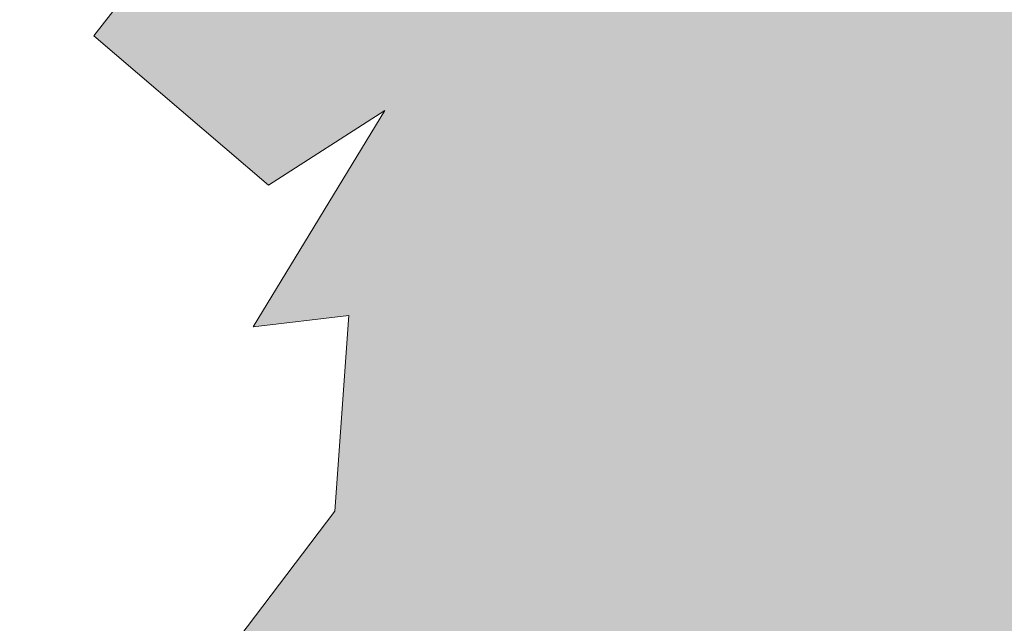
# Model space of a CAD drawing. Units: inches. Extents: x 2091 to 2899, y 967 to 2217.
# Tile 256 of 256: x 2231.62 to 2253.52, y 1152.59 to 1166.02. Entities that reach past the tile are written whole.
import ezdxf

# ---------------------------------------------------------------- set-up
doc = ezdxf.new("R2010")
doc.units = ezdxf.units.IN
doc.layers.add('A-ANNO-DIMS', color=2, linetype='Continuous', lineweight=18)
doc.layers.add('L-PLNT-TREE', color=94, linetype='Continuous', lineweight=13)
doc.layers.add('A-WALL-PATT', color=141, linetype='Continuous', lineweight=13, true_color=0xadddf7)
doc.layers.add('L-PLNT-PATT', color=114, linetype='Continuous', lineweight=13, true_color=0x139b48)
doc.styles.get("Standard").update_dxf_attribs({"font": 'arial.ttf'})
doc.dimstyles.new('ISO-25', dxfattribs={"dimtxt": 4, "dimasz": 4, "dimexe": 1.25, "dimexo": 0.625, "dimtad": 1, "dimdec": 0, "dimlunit": 3, "dimtxsty": 'Standard', "dimcen": 2.5, "dimadec": 0, "dimazin": 0, "dimtfac": 1, "dimtdec": 0, "dimtmove": 0, "dimatfit": 3, "dimfxl": 1, "dimarcsym": 0})

# ---------------------------------------------------------------- blocks, each defined once
blk = doc.blocks.new('*U25')
blk.add_lwpolyline([(-1139.42368, 1783.79628), (-1216.11644, 1685.47796), (-1117.5111, 1601.2033), (-1051.7759, 1643.3419), (-1126.09884, 1521.20092), (-1072.10606, 1527.49758), (-1079.90386, 1416.93646), (-1259.93906, 1179.83508), (-1479.05978, 1165.78888), (-1577.66258, 1109.60662), (-1742.00312, 927.01364), (-1676.26538, 814.64658), (-1270.89408, 828.69278), (-1194.20386, 772.51052), (-1007.95074, 856.78518), (-876.4778, 575.87134), (-821.70016, 575.87134), (-569.71184, 884.87504)])
blk = doc.blocks.new('*D71')
at = {"layer": 'A-ANNO-DIMS', "color": 0, "lineweight": -2, "transparency": 16777216}
for p, q in [((2212.144, 1351.294), (2212.144, 969.464)), ((2452.144, 1351.294), (2452.144, 969.464)), ((2216.144, 970.714), (2448.144, 970.714))]:
    blk.add_line(p, q, dxfattribs=at)
at = {"layer": 'A-ANNO-DIMS', "color": 0, "transparency": 16777216}
for points in [[(2216.144, 971.381), (2216.144, 970.048), (2212.144, 970.714)], [(2448.144, 971.381), (2448.144, 970.048), (2452.144, 970.714)]]:
    blk.add_solid(points, dxfattribs=at)
at = {"layer": 'Defpoints', "color": 0, "transparency": 16777216}
for p in [(2212.144, 1351.919), (2452.144, 1351.919), (2452.144, 970.714)]:
    blk.add_point(p, dxfattribs=at)
at = {"layer": 'A-ANNO-DIMS', "color": 0, "transparency": 16777216, "insert": (2332.144, 973.382), "char_height": 4, "attachment_point": 5}
blk.add_mtext('20\'-0"', dxfattribs=at)
blk = doc.blocks.new('*D75')
at = {"layer": 'A-ANNO-DIMS', "color": 0, "lineweight": -2, "transparency": 16777216}
for p, q in [((2212.144, 1274.794), (2212.144, 969.464)), ((2308.144, 1274.794), (2308.144, 969.464)), ((2216.144, 970.714), (2304.144, 970.714))]:
    blk.add_line(p, q, dxfattribs=at)
at = {"layer": 'A-ANNO-DIMS', "color": 0, "transparency": 16777216}
for points in [[(2216.144, 971.381), (2216.144, 970.048), (2212.144, 970.714)], [(2304.144, 971.381), (2304.144, 970.048), (2308.144, 970.714)]]:
    blk.add_solid(points, dxfattribs=at)
at = {"layer": 'Defpoints', "color": 0, "transparency": 16777216}
for p in [(2212.144, 1275.419), (2308.144, 1275.419), (2308.144, 970.714)]:
    blk.add_point(p, dxfattribs=at)
at = {"layer": 'A-ANNO-DIMS', "color": 0, "transparency": 16777216, "insert": (2260.144, 973.382), "char_height": 4, "attachment_point": 5}
blk.add_mtext('8\'-0"', dxfattribs=at)

msp = doc.modelspace()

# ---------------------------------------------------------------- hatches: boundary and pattern name
at = {"layer": 'A-WALL-PATT'}
h = msp.add_hatch(color=256, dxfattribs=at)
h.dxf.hatch_style = 1
h.paths.add_polyline_path([(2803.144, 2050.919), (2203.144, 2050.919), (2203.144, 1090.919), (2803.144, 1090.919)])
h.paths.add_polyline_path([(2635.799, 1147.54), (2674.524, 1147.54, 0.376086), (2678.53, 1152.88), (2678.53, 1159.556, 0.333335), (2674.524, 1163.562), (2674.524, 1163.562), (2674.524, 1192.934), (2635.806, 1192.934), (2597.088, 1192.934), (2597.088, 1163.562, 0.333335), (2593.082, 1159.556), (2593.082, 1152.88, 0.376086), (2597.088, 1147.54)], flags=0)
h.paths.add_polyline_path([(2436.01, 1278.241, 0.000483), (2435.953, 1278.215, -0.001328), (2435.936, 1278.112, -0.001711), (2436.116, 1278.041, 0.002185)], flags=0)
h.paths.add_polyline_path([(2794.144, 1143.419), (2794.144, 1347.419), (2543.37, 1347.419), (2543.37, 1351.919), (2794.144, 1351.919), (2794.144, 1392.714), (2793.947, 1392.714), (2793.947, 1473.537), (2794.144, 1473.537), (2794.144, 1531.919), (2650.144, 1531.919), (2650.144, 1536.419), (2794.144, 1536.419), (2794.144, 1692.419), (2609.376, 1692.419), (2609.376, 1644.419), (2604.876, 1644.419), (2604.876, 1744.919), (2609.376, 1744.919), (2609.376, 1696.919), (2794.144, 1696.919), (2794.144, 1780.919), (2609.644, 1780.919), (2493.876, 1780.919), (2493.876, 1785.419), (2609.644, 1785.419), (2794.144, 1785.419), (2794.144, 1847.939), (2793.951, 1847.939), (2793.951, 1928.762), (2794.144, 1928.762), (2794.144, 1941.419), (2614.144, 1941.419), (2614.144, 1821.419), (2609.644, 1821.419), (2609.644, 1941.419), (2392.144, 1941.419), (2392.144, 1819.919), (2387.644, 1819.919), (2387.644, 1941.419), (2212.144, 1941.419), (2212.144, 1783.919), (2392.144, 1783.919), (2392.144, 1780.919), (2212.144, 1780.919), (2212.144, 1629.419), (2387.644, 1629.419), (2387.644, 1744.919), (2392.144, 1744.919), (2392.144, 1627.919), (2317.144, 1627.919), (2317.144, 1551.419), (2317.144, 1536.419), (2459.384, 1536.419), (2459.384, 1602.396), (2463.884, 1602.396), (2463.884, 1531.919), (2456.644, 1531.919), (2456.644, 1529.919), (2452.144, 1529.919), (2452.144, 1531.919), (2312.644, 1531.919), (2312.644, 1551.419), (2306.144, 1551.419), (2306.144, 1555.919), (2308.144, 1555.919), (2308.144, 1551.419), (2312.644, 1551.419), (2312.644, 1627.919), (2212.144, 1627.919), (2212.144, 1555.919), (2270.144, 1555.919), (2270.144, 1551.419), (2212.144, 1551.419), (2212.144, 1351.919), (2272.144, 1351.919), (2272.144, 1347.419), (2212.144, 1347.419), (2212.144, 1275.419), (2308.144, 1275.419), (2308.144, 1351.919), (2452.144, 1351.919), (2452.144, 1493.919), (2456.644, 1493.919), (2456.644, 1347.419), (2312.644, 1347.419), (2312.644, 1270.919), (2212.144, 1270.919), (2212.144, 1099.919), (2281.238, 1099.919), (2282.871, 1110.914), (2282.008, 1116.997), (2278.558, 1121.42), (2268.206, 1128.056), (2272.088, 1128.056), (2273.813, 1131.927), (2279.42, 1134.692), (2285.028, 1135.245), (2287.616, 1137.457), (2288.047, 1138.01), (2289.341, 1140.775), (2291.067, 1139.669), (2292.361, 1135.245), (2295.38, 1136.904), (2296.243, 1135.798), (2297.105, 1133.033), (2300.125, 1138.01), (2303.144, 1138.01), (2304.438, 1135.798), (2303.144, 1133.586), (2306.595, 1134.692), (2307.889, 1133.033), (2310.908, 1135.245), (2313.927, 1134.139), (2315.627, 1132.427), (2308.32, 1117.55), (2290.204, 1109.808), (2288.91, 1103.172), (2289.272, 1099.919), (2434.918, 1099.919), (2431.593, 1124.788), (2429.93, 1169.553), (2430.927, 1240.52), (2435.659, 1238.186), (2437.135, 1196.554), (2438.798, 1143.973), (2442.678, 1111.998), (2446.558, 1099.919), (2794.144, 1099.919), (2794.144, 1138.919), (2548.032, 1138.919), (2548.032, 1143.419), (2548.032, 1148.819), (2546.668, 1148.032), (2528.686, 1179.179, 0.256256), (2512.032, 1148.819), (2512.032, 1143.419), (2512.032, 1138.919), (2507.532, 1138.919), (2507.532, 1143.419), (2507.532, 1148.819, 0.256256), (2490.879, 1179.179), (2472.896, 1148.032), (2471.532, 1148.819), (2471.532, 1143.419), (2467.032, 1143.419), (2467.032, 1269.946, 0.039061), (2460.91, 1273.58), (2467.032, 1273.58), (2467.032, 1286.325, 0.014511), (2465.216, 1286.762), (2467.032, 1287.053), (2467.032, 1323.419), (2471.532, 1323.419), (2471.532, 1148.819), (2489.532, 1179.996), (2490.896, 1179.208), (2490.879, 1179.179, -0.256256), (2507.532, 1148.819), (2507.532, 1143.419), (2512.032, 1143.419), (2512.032, 1148.819, -0.256256), (2528.686, 1179.179), (2528.668, 1179.208), (2530.032, 1179.996), (2548.032, 1148.819), (2548.032, 1143.419)], flags=16)
h.paths.add_polyline_path([(2607.769, 1200.945), (2607.769, 1265.031), (2597.088, 1281.052), (2619.785, 1281.052), (2627.795, 1337.127), (2635.799, 1337.127), (2643.817, 1337.127), (2651.827, 1281.052), (2674.524, 1281.052), (2663.843, 1265.031), (2663.843, 1200.945), (2635.806, 1200.945)], flags=0)
edge = h.paths.add_edge_path(flags=0)
edge.add_ellipse((13303.896, 1272.999), major_axis=(-10595.313, 0), ratio=0.84230387, start_angle=0.6282372, end_angle=0.6465541, ccw=False)
edge.add_ellipse((2711.7, 1156.853), major_axis=(2.22, 0), ratio=0.842304, start_angle=111.5352, end_angle=180.6282, ccw=False)
edge.add_ellipse((13303.156, 1272.999), major_axis=(-10593.026, 0), ratio=0.84230387, start_angle=0.5282715, end_angle=0.6465541, ccw=False)
edge.add_line((2710.765, 1175.333), (2710.13, 1175.333))
edge.add_ellipse((2710.13, 1176.58), major_axis=(1.48, 0), ratio=0.842304, start_angle=180, end_angle=270, ccw=False)
edge.add_line((2708.65, 1176.58), (2708.65, 1200.783))
edge.add_ellipse((2710.13, 1200.783), major_axis=(1.48, 0), ratio=0.842304, start_angle=90, end_angle=180, ccw=False)
edge.add_line((2710.13, 1202.029), (2710.465, 1202.029))
edge.add_ellipse((13303.156, 1272.999), major_axis=(-10593.026, 0), ratio=0.84230387, start_angle=-0.0902291, end_angle=0.3838668, ccw=False)
edge.add_ellipse((2710.13, 1290.927), major_axis=(-1.48, 0), ratio=0.842304, start_angle=0, end_angle=90, ccw=False)
edge.add_line((2708.65, 1290.927), (2708.65, 1315.13))
edge.add_ellipse((2710.13, 1315.13), major_axis=(-1.48, 0), ratio=0.842304, start_angle=-90, end_angle=0, ccw=False)
edge.add_line((2710.13, 1316.377), (2710.706, 1316.377))
edge.add_ellipse((3238.402, 1296.29), major_axis=(528.234, 0), ratio=0.8423039, start_angle=176.34957, end_angle=177.82005, ccw=False)
edge.add_ellipse((2775.063, 1071.451), major_axis=(313.308, 0), ratio=0.8423039, start_angle=102.12597, end_angle=103.78053, ccw=False)
edge.add_ellipse((2775.063, 1078.306), major_axis=(-305.303, 0), ratio=0.8423039, start_angle=-79.79046, end_angle=-77.55537, ccw=False)
edge.add_ellipse((2695.142, 1541.975), major_axis=(-250.96, 0), ratio=0.8423039, start_angle=99.25657, end_angle=102.55493)
edge.add_line((2741.41, 1334.214), (2747.133, 1337.378))
edge.add_ellipse((2747.539, 1336.857), major_axis=(-0.74, 0), ratio=0.842304, start_angle=270, end_angle=307.9331, ccw=False)
edge.add_ellipse((2747.539, 1336.857), major_axis=(-0.74, 0), ratio=0.842304, start_angle=232.0669, end_angle=270, ccw=False)
edge.add_line((2747.945, 1337.378), (2753.667, 1334.214))
edge.add_ellipse((2799.935, 1541.975), major_axis=(250.96, 0), ratio=0.8423039, start_angle=257.44507, end_angle=260.74343)
edge.add_ellipse((2720.014, 1078.306), major_axis=(305.303, 0), ratio=0.8423039, start_angle=77.55537, end_angle=79.79046, ccw=False)
edge.add_ellipse((2720.014, 1071.451), major_axis=(-313.308, 0), ratio=0.8423039, start_angle=256.21947, end_angle=257.87403, ccw=False)
edge.add_ellipse((2256.676, 1296.29), major_axis=(-528.234, 0), ratio=0.8423039, start_angle=182.17995, end_angle=183.65043, ccw=False)
edge.add_line((2784.371, 1316.377), (2784.947, 1316.377))
edge.add_ellipse((2784.947, 1315.13), major_axis=(1.48, 0), ratio=0.842304, start_angle=0, end_angle=90, ccw=False)
edge.add_line((2786.427, 1315.13), (2786.427, 1290.927))
edge.add_ellipse((2784.947, 1290.927), major_axis=(1.48, 0), ratio=0.842304, start_angle=270, end_angle=360, ccw=False)
edge.add_ellipse((-7808.079, 1272.999), major_axis=(10593.026, 0), ratio=0.84230387, start_angle=-0.3838668, end_angle=0.0902291, ccw=False)
edge.add_line((2784.612, 1202.029), (2784.947, 1202.029))
edge.add_ellipse((2784.947, 1200.783), major_axis=(1.48, 0), ratio=0.842304, start_angle=0, end_angle=90, ccw=False)
edge.add_line((2786.427, 1200.783), (2786.427, 1176.58))
edge.add_ellipse((2784.947, 1176.58), major_axis=(-1.48, 0), ratio=0.842304, start_angle=90, end_angle=180, ccw=False)
edge.add_line((2784.947, 1175.333), (2784.313, 1175.333))
edge.add_ellipse((-7808.079, 1272.999), major_axis=(10593.026, 0), ratio=0.84230387, start_angle=-0.6186432, end_angle=-0.5282715, ccw=False)
edge.add_ellipse((2783.377, 1156.853), major_axis=(-2.22, 0), ratio=0.842304, start_angle=179.3718, end_angle=248.4648, ccw=False)
edge.add_ellipse((-7808.819, 1272.999), major_axis=(-10595.313, 0), ratio=0.842303866, start_angle=179.3534459, end_angle=179.3717628, ccw=False)
edge.add_ellipse((2780.297, 1153.501), major_axis=(-5.246, 0), ratio=0.842304, start_angle=90, end_angle=179.3534, ccw=False)
edge.add_line((2780.297, 1149.082), (2714.78, 1149.082))
edge.add_ellipse((2714.78, 1153.501), major_axis=(5.246, 0), ratio=0.842304, start_angle=180.6466, end_angle=270, ccw=False)
edge = h.paths.add_edge_path(flags=0)
edge.add_line((2718.187, 1151.008), (2718.187, 1170.472))
edge.add_ellipse((2721.147, 1170.472), major_axis=(-2.96, 0), ratio=0.842304, start_angle=-90, end_angle=0, ccw=False)
edge.add_line((2721.147, 1172.965), (2773.93, 1172.965))
edge.add_ellipse((2773.93, 1170.472), major_axis=(-2.96, 0), ratio=0.842304, start_angle=180, end_angle=270, ccw=False)
edge.add_line((2776.89, 1170.472), (2776.89, 1151.008))
edge.add_line((2776.89, 1151.008), (2718.187, 1151.008))
edge = h.paths.add_edge_path(flags=0)
edge.add_line((2718.187, 1180.234), (2718.187, 1199.058))
edge.add_ellipse((2747.539, 1320.399), major_axis=(147.018, 0), ratio=0.8423039, start_angle=256.40187, end_angle=283.59813)
edge.add_line((2776.89, 1199.058), (2776.89, 1180.234))
edge.add_ellipse((2747.539, 1301.575), major_axis=(147.018, 0), ratio=0.8423039, start_angle=256.40187, end_angle=283.59813, ccw=False)
edge = h.paths.add_edge_path(flags=0)
edge.add_ellipse((13303.156, 1272.999), major_axis=(-10591.546, 0), ratio=0.84230387, start_angle=0.0555943, end_angle=0.3777642, ccw=False)
edge.add_line((2711.617, 1262.722), (2715.667, 1249.495))
edge.add_ellipse((6413.892, 1241.692), major_axis=(-3698.236, 0), ratio=0.84230387, start_angle=-0.120897, end_angle=0.364076)
edge.add_line((2715.761, 1218.192), (2711.934, 1203.167))
edge = h.paths.add_edge_path(flags=0)
edge.add_line((2718.187, 1251.075), (2716.002, 1267.45))
edge.add_ellipse((2742.151, 1202.19), major_axis=(81.773, 0), ratio=0.842304, start_angle=94.27742, end_angle=111.83495, ccw=False)
edge.add_line((2737.01, 1270.931), (2758.067, 1270.931))
edge.add_ellipse((2752.926, 1202.19), major_axis=(81.773, 0), ratio=0.842304, start_angle=68.16505, end_angle=85.72258, ccw=False)
edge.add_line((2779.075, 1267.45), (2776.89, 1251.075))
edge.add_ellipse((2750.338, 1187.885), major_axis=(79.58, 0), ratio=0.842304, start_angle=67.20809, end_angle=85.12993)
edge.add_line((2756.035, 1254.744), (2739.043, 1254.744))
edge.add_ellipse((2744.739, 1187.885), major_axis=(79.58, 0), ratio=0.842304, start_angle=94.87007, end_angle=112.79191)
edge = h.paths.add_edge_path(flags=0)
edge.add_line((2783.143, 1203.167), (2779.316, 1218.192))
edge.add_ellipse((-918.815, 1241.692), major_axis=(3698.236, 0), ratio=0.84230387, start_angle=-0.364076, end_angle=0.120897)
edge.add_line((2779.41, 1249.495), (2783.46, 1262.722))
edge.add_ellipse((-7808.079, 1272.999), major_axis=(-10591.546, 0), ratio=0.84230387, start_angle=179.6222358, end_angle=179.9444057, ccw=False)
edge = h.paths.add_edge_path(flags=0)
edge.add_ellipse((2734.201, 1286.69), major_axis=(-0.357, 6.34), ratio=0.603834, start_angle=89.002, end_angle=253.6574, ccw=False)
edge.add_line((2730.369, 1286.542), (2730.369, 1301.352))
edge.add_line((2730.369, 1301.352), (2735.913, 1305.215))
edge.add_ellipse((2736.385, 1304.735), major_axis=(0.74, 0), ratio=0.842304, start_angle=90, end_angle=134.4802, ccw=False)
edge.add_line((2736.385, 1305.358), (2738.033, 1305.358))
edge.add_line((2738.033, 1305.358), (2738.033, 1307.708))
edge.add_ellipse((2794.202, 1307.708), major_axis=(56.169, 0), ratio=0.842304, start_angle=150.5614, end_angle=180, ccw=False)
edge.add_ellipse((2700.876, 1307.708), major_axis=(-56.169, 0), ratio=0.842304, start_angle=180, end_angle=209.4386, ccw=False)
edge.add_line((2757.044, 1307.708), (2757.044, 1305.358))
edge.add_line((2757.044, 1305.358), (2758.692, 1305.358))
edge.add_ellipse((2758.692, 1304.735), major_axis=(-0.74, 0), ratio=0.842304, start_angle=225.5198, end_angle=270, ccw=False)
edge.add_line((2759.164, 1305.215), (2764.708, 1301.352))
edge.add_line((2764.708, 1301.352), (2764.708, 1286.542))
edge.add_ellipse((2760.876, 1286.69), major_axis=(0.357, 6.34), ratio=0.603834, start_angle=106.3426, end_angle=270.998, ccw=False)
edge.add_line((2757.044, 1285.797), (2757.044, 1307.708))
edge.add_ellipse((2700.876, 1307.708), major_axis=(-56.169, 0), ratio=0.842304, start_angle=180, end_angle=209.4386)
edge.add_ellipse((2794.202, 1307.708), major_axis=(56.169, 0), ratio=0.842304, start_angle=150.5614, end_angle=180)
edge.add_line((2738.033, 1307.708), (2738.033, 1285.797))
h.paths.add_polyline_path([(2417.812, 1104.45), (2413.492, 1102.53), (2410.612, 1103.97), (2409.172, 1106.37), (2407.252, 1107.33), (2406.292, 1109.73), (2405.332, 1114.05), (2405.332, 1117.89), (2406.292, 1120.13), (2407.252, 1119.81), (2408.848, 1118.328), (2410.174, 1119.424), (2410.211, 1120.406), (2411.041, 1121.419), (2410.699, 1119.859), (2410.174, 1119.424), (2410.088, 1117.176), (2411.133, 1116.206), (2413.972, 1119.33), (2416.852, 1120.77), (2416.87, 1120.799), (2417.035, 1119.405), (2417.896, 1118.143), (2418.292, 1118.37), (2419.544, 1120.039), (2419.361, 1118.387), (2419.032, 1119.356), (2418.399, 1118.512), (2419.252, 1114.53), (2418.794, 1107.199)], flags=0)
h.paths.add_polyline_path([(2508.87, 1347.419), (2508.37, 1347.419), (2508.37, 1351.919), (2508.87, 1351.919)], flags=0)
h.paths.add_polyline_path([(2473.37, 1347.419), (2472.37, 1347.419), (2467.87, 1347.419), (2467.87, 1455.419), (2472.37, 1455.419), (2472.37, 1352.419), (2473.37, 1352.419)], flags=0)
h.paths.add_polyline_path([(2352.106, 1217.446), (2349.226, 1218.886), (2347.786, 1221.286), (2345.866, 1222.246), (2344.906, 1224.646), (2343.946, 1228.966), (2343.946, 1232.806), (2344.906, 1235.046), (2345.866, 1234.726), (2347.462, 1233.244), (2348.788, 1234.341), (2348.825, 1235.322), (2349.655, 1236.336), (2349.313, 1234.775), (2348.788, 1234.341), (2348.702, 1232.093), (2349.747, 1231.123), (2352.586, 1234.246), (2355.466, 1235.686), (2355.484, 1235.715), (2355.649, 1234.322), (2356.51, 1233.06), (2356.906, 1233.286), (2358.158, 1234.956), (2357.975, 1233.304), (2357.646, 1234.273), (2357.013, 1233.428), (2357.866, 1229.446), (2357.408, 1222.115), (2356.426, 1219.366)], flags=0)
h.paths.add_polyline_path([(2348.297, 1112.224), (2347.014, 1112.31), (2345.53, 1114.127), (2345.732, 1115.858), (2346.812, 1116.982), (2346.812, 1114.646), (2345.867, 1114.214), (2346.88, 1114.3)], flags=0)
h.paths.add_polyline_path([(2347.014, 1110.926), (2346.272, 1110.493), (2346.61, 1111.186)], flags=0)
h.paths.add_polyline_path([(2345.867, 1118.194), (2345.53, 1117.329), (2343.708, 1118.021), (2344.383, 1118.626)], flags=0)
h.paths.add_polyline_path([(2346.677, 1109.282), (2346.07, 1108.071), (2345.867, 1110.061)], flags=0)
h.paths.add_polyline_path([(2345.057, 1119.751), (2343.64, 1119.751), (2343.978, 1121.135)], flags=0)
h.paths.add_polyline_path([(2345.26, 1116.55), (2345.125, 1115.858), (2344.922, 1115.685), (2344.72, 1116.377)], flags=0)
h.paths.add_polyline_path([(2345.665, 1112.31), (2345.462, 1111.532), (2344.045, 1111.964), (2344.652, 1112.57)], flags=0)
h.paths.add_polyline_path([(2345.192, 1113.349), (2344.45, 1113.868), (2344.72, 1114.387)], flags=0)
h.paths.add_polyline_path([(2344.652, 1116.809), (2344.18, 1115.685), (2344.652, 1115.339), (2343.91, 1114.906), (2343.033, 1115.944), (2343.64, 1116.463)], flags=0)
h.paths.add_polyline_path([(2345.867, 1106.686), (2344.99, 1105.562), (2344.517, 1106.6)], flags=0)
h.paths.add_polyline_path([(2344.855, 1110.061), (2344.517, 1109.282), (2344.113, 1109.715)], flags=0)
h.paths.add_polyline_path([(2344.045, 1113.522), (2343.438, 1113.089), (2342.763, 1113.954)], flags=0)
h.paths.add_polyline_path([(2344.315, 1111.012), (2342.965, 1110.32), (2342.965, 1111.099)], flags=0)
h.paths.add_polyline_path([(2345.125, 1104.697), (2344.585, 1103.745), (2344.45, 1104.264)], flags=0)
h.paths.add_polyline_path([(2342.83, 1121.222), (2341.75, 1120.53), (2340.536, 1121.049), (2340.131, 1121.828), (2340.671, 1122.952), (2341.143, 1121.828), (2341.615, 1122.001)], flags=0)
h.paths.add_polyline_path([(2342.965, 1119.751), (2343.033, 1118.453), (2342.088, 1118.021), (2342.02, 1119.491)], flags=0)
h.paths.add_polyline_path([(2342.695, 1116.896), (2341.953, 1116.636), (2342.02, 1117.329)], flags=0)
h.paths.add_polyline_path([(2343.033, 1112.224), (2342.02, 1111.791), (2341.548, 1112.224), (2342.358, 1113.349)], flags=0)
h.paths.add_polyline_path([(2343.775, 1104.437), (2342.628, 1102.88), (2342.695, 1104.61), (2343.438, 1105.129)], flags=0)
h.paths.add_polyline_path([(2342.02, 1115.079), (2340.806, 1115.512), (2340.941, 1116.377)], flags=0)
h.paths.add_polyline_path([(2341.481, 1120.097), (2341.481, 1119.405), (2341.076, 1119.578), (2341.143, 1120.097)], flags=0)
h.paths.add_polyline_path([(2341.818, 1114.473), (2340.941, 1113.089), (2340.806, 1114.56)], flags=0)
h.paths.add_polyline_path([(2341.143, 1118.54), (2340.941, 1116.982), (2339.051, 1117.675), (2339.051, 1118.626)], flags=0)
h.paths.add_polyline_path([(2342.695, 1101.668), (2341.953, 1101.841), (2342.56, 1102.361)], flags=0)
h.paths.add_polyline_path([(2340.333, 1119.665), (2338.444, 1119.578), (2337.904, 1120.357), (2339.658, 1120.616)], flags=0)
h.paths.add_polyline_path([(2340.333, 1115.339), (2340.063, 1113.695), (2339.388, 1115.339)], flags=0)
h.paths.add_polyline_path([(2341.818, 1103.831), (2341.548, 1102.88), (2341.143, 1103.658)], flags=0)
h.paths.add_polyline_path([(2339.051, 1122.866), (2337.296, 1121.828), (2337.094, 1123.125), (2337.769, 1123.818)], flags=0)
h.paths.add_polyline_path([(2339.118, 1121.741), (2338.848, 1121.222), (2338.174, 1121.049), (2338.376, 1121.568)], flags=0)
h.paths.add_polyline_path([(2339.186, 1119.319), (2338.646, 1118.713), (2338.241, 1118.107), (2338.241, 1118.886)], flags=0)
h.paths.add_polyline_path([(2341.143, 1101.928), (2340.603, 1101.236), (2340.063, 1101.841), (2340.603, 1102.361)], flags=0)
h.paths.add_polyline_path([(2337.634, 1117.761), (2336.621, 1118.28), (2337.296, 1118.972)], flags=0)
h.paths.add_polyline_path([(2336.824, 1119.578), (2334.799, 1118.972), (2335.204, 1120.357), (2336.554, 1120.876)], flags=0)
h.paths.add_polyline_path([(2339.118, 1100.457), (2337.364, 1100.543), (2336.756, 1101.236)], flags=0)
h.paths.add_polyline_path([(2336.351, 1122.433), (2336.014, 1121.914), (2334.934, 1122.433), (2334.529, 1123.471), (2335.744, 1122.779)], flags=0)
h.paths.add_polyline_path([(2334.732, 1120.876), (2334.259, 1120.357), (2334.057, 1120.789), (2334.597, 1121.308)], flags=0)
h.paths.add_polyline_path([(2334.462, 1122.174), (2332.572, 1121.308), (2331.357, 1122.174), (2332.1, 1122.866)], flags=0)
h.paths.add_polyline_path([(2334.259, 1118.54), (2333.382, 1118.453), (2333.652, 1119.319)], flags=0)
h.paths.add_polyline_path([(2335.542, 1102.274), (2334.192, 1102.62), (2335.272, 1103.312)], flags=0)
h.paths.add_polyline_path([(2332.707, 1119.665), (2331.695, 1120.443), (2332.505, 1120.789)], flags=0)
h.paths.add_polyline_path([(2334.732, 1101.149), (2333.517, 1101.582), (2333.989, 1101.755)], flags=0)
h.paths.add_polyline_path([(2332.64, 1116.636), (2331.087, 1116.29), (2331.965, 1118.194)], flags=0)
h.paths.add_polyline_path([(2330.75, 1121.568), (2330.277, 1120.27), (2328.523, 1119.319), (2328.995, 1121.049)], flags=0)
h.paths.add_polyline_path([(2330.75, 1118.626), (2330.008, 1117.502), (2329.873, 1118.021)], flags=0)
h.paths.add_polyline_path([(2332.1, 1102.361), (2330.547, 1102.014), (2331.695, 1102.966)], flags=0)
h.paths.add_polyline_path([(2329.535, 1113.608), (2329.063, 1112.31), (2328.59, 1113.349)], flags=0)
h.paths.add_polyline_path([(2328.388, 1117.848), (2327.51, 1116.55), (2327.173, 1117.761)], flags=0)
h.paths.add_polyline_path([(2329.738, 1106.513), (2329.535, 1105.302), (2328.253, 1106.081)], flags=0)
h.paths.add_polyline_path([(2328.658, 1114.387), (2328.05, 1114.127), (2328.32, 1114.906)], flags=0)
h.paths.add_polyline_path([(2328.32, 1112.224), (2327.106, 1112.137), (2326.701, 1112.656)], flags=0)
h.paths.add_polyline_path([(2326.903, 1115.252), (2326.701, 1114.127), (2325.216, 1113.608), (2326.093, 1115.339)], flags=0)
h.paths.add_polyline_path([(2326.633, 1108.33), (2326.093, 1107.379), (2325.891, 1108.503), (2326.498, 1109.109)], flags=0)
h.paths.add_polyline_path([(2615.144, 1531.919), (2609.644, 1531.919), (2609.644, 1620.419), (2614.144, 1620.419), (2614.144, 1536.419), (2615.144, 1536.419)], flags=0)
h.paths.add_polyline_path([(2545.144, 1563.419), (2464.144, 1563.419), (2464.144, 1632.419), (2509.144, 1632.419), (2509.144, 1627.919), (2509.144, 1603.919), (2468.644, 1603.919), (2468.644, 1567.919), (2540.644, 1567.919), (2540.644, 1591.919), (2545.144, 1591.919)], flags=0)
h.paths.add_polyline_path([(2388.969, 1549.986), (2357.434, 1549.986), (2357.434, 1623.361), (2399.363, 1623.361), (2435.689, 1623.361), (2435.593, 1602.559), (2435.593, 1602.396), (2388.969, 1602.396)], flags=0)
h.paths.add_polyline_path([(2388.881, 1555.809), (2374.904, 1555.809), (2374.904, 1600.572), (2374.904, 1615.458), (2406.351, 1615.458), (2406.351, 1618.939), (2412.174, 1615.458), (2406.351, 1611.976), (2406.351, 1615.458), (2388.881, 1615.458)], flags=0)
h.paths.add_polyline_path([(2568.876, 1644.419), (2453.376, 1644.419), (2453.376, 1785.419), (2457.876, 1785.419), (2457.876, 1648.919), (2568.876, 1648.919)], flags=0)
h.paths.add_polyline_path([(2212.144, 1945.919), (2212.144, 2041.919), (2794.144, 2041.919), (2794.144, 1945.919)], flags=16)
h.paths.add_polyline_path([(2271.083, 1964.317), (2776.853, 1964.317), (2776.853, 2037.17), (2271.083, 2037.17)], flags=8)
h.paths.add_polyline_path([(2380.649, 1536.824), (2461.041, 1536.824), (2461.041, 1554.653), (2380.649, 1554.653)], flags=8)
h.paths.add_polyline_path([(2240.756, 1609.725), (2309.186, 1609.725), (2309.186, 1617.698), (2240.756, 1617.698)], flags=8)
h.paths.add_polyline_path([(2212.677, 1313.504), (2282.592, 1313.504), (2282.592, 1322.745), (2212.677, 1322.745)], flags=8)
h.paths.add_polyline_path([(2457.112, 1114.779), (2558.482, 1114.779), (2558.482, 1142.22), (2457.112, 1142.22)], flags=8)
h.paths.add_polyline_path([(2473.442, 1273.01), (2604.641, 1273.01), (2604.641, 1318.347), (2473.442, 1318.347)], flags=8)
h.paths.add_polyline_path([(2638.876, 1626.977), (2684.25, 1627.977), (2684.038, 1637.597), (2638.664, 1636.598)], flags=8)
h.paths.add_polyline_path([(2537.591, 1453.793), (2628.39, 1453.793), (2628.39, 1475.345), (2537.591, 1475.345)], flags=8)
h.paths.add_polyline_path([(2504.138, 1714.632), (2554.647, 1714.632), (2554.647, 1730.238), (2504.138, 1730.238)], flags=8)
h.paths.add_polyline_path([(2487.501, 1575.652), (2535.097, 1575.652), (2535.097, 1598.378), (2487.501, 1598.378)], flags=8)
h.paths.add_polyline_path([(2709.099, 1735.71), (2740.017, 1735.71), (2740.017, 1749.938), (2709.099, 1749.938)], flags=8)
h.paths.add_polyline_path([(2442.438, 1792.172), (2564.729, 1792.172), (2564.729, 1842), (2442.438, 1842)], flags=8)
h.paths.add_polyline_path([(2655.816, 1809.644), (2789.52, 1806.694), (2790.085, 1832.292), (2656.381, 1835.242)], flags=8)
h.paths.add_polyline_path([(2234.843, 1797.72), (2368.593, 1794.769), (2369.161, 1820.504), (2235.411, 1823.455)], flags=8)
h.paths.add_polyline_path([(2245.138, 1644.006), (2398.428, 1640.624), (2398.995, 1666.325), (2245.706, 1669.707)], flags=8)
h.paths.add_polyline_path([(2306.143, 1431.169), (2413.768, 1428.794), (2414.333, 1454.392), (2306.708, 1456.766)], flags=8)
h.paths.add_polyline_path([(2306.835, 1458.233), (2393.38, 1456.323), (2393.933, 1481.354), (2307.387, 1483.264)], flags=8)
at = {"layer": 'L-PLNT-PATT'}
h = msp.add_hatch(color=256, dxfattribs=at)
h.dxf.hatch_style = 1
h.paths.add_polyline_path([(2333.338, 1165.659), (2329.024, 1166.212), (2331.612, 1168.424), (2335.063, 1177.271), (2328.162, 1184.46), (2319.535, 1187.225), (2323.417, 1193.308), (2319.966, 1203.814), (2317.809, 1203.814), (2313.496, 1213.215), (2310.908, 1212.662), (2307.889, 1212.662), (2305.732, 1217.086), (2307.026, 1223.168), (2310.477, 1223.168), (2304.007, 1230.91), (2303.136, 1237.046), (2299.693, 1240.864), (2296.674, 1237.546), (2294.949, 1238.652), (2294.517, 1241.417), (2292.361, 1242.523), (2289.341, 1239.758), (2285.89, 1240.311), (2283.302, 1235.334), (2283.302, 1230.91), (2286.753, 1229.251), (2284.165, 1227.592), (2281.577, 1229.804), (2274.244, 1222.615), (2274.244, 1220.957), (2271.225, 1219.298), (2272.088, 1217.639), (2274.244, 1214.321), (2270.362, 1211.556), (2266.48, 1214.321), (2264.324, 1213.768), (2263.461, 1211.556), (2266.48, 1211.003), (2266.912, 1206.579), (2263.539, 1207.132), (2259.579, 1203.261), (2263.892, 1202.708), (2262.167, 1197.178), (2258.285, 1196.625), (2253.971, 1193.861), (2248.795, 1191.096), (2248.364, 1193.308), (2244.482, 1185.013), (2251.383, 1186.672), (2255.697, 1183.907), (2254.403, 1177.271), (2246.639, 1174.506), (2243.188, 1176.718), (2241.894, 1173.4), (2238.875, 1172.847), (2236.287, 1169.53), (2233.267, 1165.659), (2237.149, 1162.341), (2239.737, 1164), (2236.811, 1159.191), (2238.937, 1159.439), (2238.63, 1155.086), (2231.542, 1145.752), (2222.915, 1145.199), (2219.033, 1142.987), (2212.563, 1135.798), (2215.151, 1131.374), (2231.111, 1131.927), (2234.13, 1129.715), (2241.463, 1133.033), (2246.639, 1121.973), (2248.795, 1121.973), (2258.716, 1134.139), (2261.736, 1135.798), (2263.892, 1133.033), (2263.892, 1129.162), (2267.343, 1128.056), (2272.088, 1128.056), (2273.813, 1131.927), (2279.42, 1134.692), (2285.028, 1135.245), (2287.616, 1137.457), (2288.047, 1138.01), (2289.341, 1140.775), (2291.067, 1139.669), (2292.361, 1135.245), (2295.38, 1136.904), (2296.243, 1135.798), (2297.105, 1133.033), (2300.125, 1138.01), (2303.144, 1138.01), (2304.438, 1135.798), (2303.144, 1133.586), (2306.595, 1134.692), (2307.889, 1133.033), (2310.908, 1135.245), (2313.927, 1134.139), (2319.966, 1128.056), (2322.554, 1126.95), (2324.711, 1124.738), (2342.827, 1126.397), (2346.278, 1123.079), (2348.866, 1124.185), (2341.964, 1133.033), (2341.533, 1136.351), (2343.69, 1139.669), (2339.808, 1150.175), (2337.651, 1150.175)])
h.paths.add_polyline_path([(2339.658, 1120.616), (2337.904, 1120.357), (2338.444, 1119.578), (2340.333, 1119.665)])
h.paths.add_polyline_path([(2341.143, 1118.54), (2339.051, 1118.626), (2339.051, 1117.675), (2340.941, 1116.982)])
h.paths.add_polyline_path([(2336.554, 1120.876), (2335.204, 1120.357), (2334.799, 1118.972), (2336.824, 1119.578)])
h.paths.add_polyline_path([(2337.296, 1118.972), (2336.621, 1118.28), (2337.634, 1117.761)])
h.paths.add_polyline_path([(2338.646, 1118.713), (2339.186, 1119.319), (2338.241, 1118.886), (2338.241, 1118.107)])
h.paths.add_polyline_path([(2339.051, 1122.866), (2337.769, 1123.818), (2337.094, 1123.125), (2337.296, 1121.828)])
h.paths.add_polyline_path([(2341.615, 1122.001), (2341.143, 1121.828), (2340.671, 1122.952), (2340.131, 1121.828), (2340.536, 1121.049), (2341.75, 1120.53), (2342.83, 1121.222)])
h.paths.add_polyline_path([(2342.965, 1119.751), (2342.02, 1119.491), (2342.088, 1118.021), (2343.033, 1118.453)])
h.paths.add_polyline_path([(2345.867, 1118.194), (2344.383, 1118.626), (2343.708, 1118.021), (2345.53, 1117.329)])
h.paths.add_polyline_path([(2344.652, 1116.809), (2343.64, 1116.463), (2343.033, 1115.944), (2343.91, 1114.906), (2344.652, 1115.339), (2344.18, 1115.685)])
h.paths.add_polyline_path([(2346.812, 1116.982), (2345.732, 1115.858), (2345.53, 1114.127), (2347.014, 1112.31), (2348.297, 1112.224), (2346.88, 1114.3), (2345.867, 1114.214), (2346.812, 1114.646)])
h.paths.add_polyline_path([(2345.26, 1116.55), (2344.72, 1116.377), (2344.922, 1115.685), (2345.125, 1115.858)])
h.paths.add_polyline_path([(2342.695, 1116.896), (2342.02, 1117.329), (2341.953, 1116.636)])
h.paths.add_polyline_path([(2341.481, 1120.097), (2341.143, 1120.097), (2341.076, 1119.578), (2341.481, 1119.405)])
h.paths.add_polyline_path([(2343.978, 1121.135), (2343.64, 1119.751), (2345.057, 1119.751)])
h.paths.add_polyline_path([(2339.118, 1121.741), (2338.376, 1121.568), (2338.174, 1121.049), (2338.848, 1121.222)])
h.paths.add_polyline_path([(2336.351, 1122.433), (2335.744, 1122.779), (2334.529, 1123.471), (2334.934, 1122.433), (2336.014, 1121.914)])
h.paths.add_polyline_path([(2334.462, 1122.174), (2332.1, 1122.866), (2331.357, 1122.174), (2332.572, 1121.308)])
h.paths.add_polyline_path([(2334.597, 1121.308), (2334.057, 1120.789), (2334.259, 1120.357), (2334.732, 1120.876)])
h.paths.add_polyline_path([(2332.505, 1120.789), (2331.695, 1120.443), (2332.707, 1119.665)])
h.paths.add_polyline_path([(2333.652, 1119.319), (2333.382, 1118.453), (2334.259, 1118.54)])
h.paths.add_polyline_path([(2331.965, 1118.194), (2331.087, 1116.29), (2332.64, 1116.636)])
h.paths.add_polyline_path([(2330.75, 1121.568), (2328.995, 1121.049), (2328.523, 1119.319), (2330.277, 1120.27)])
h.paths.add_polyline_path([(2330.75, 1118.626), (2329.873, 1118.021), (2330.008, 1117.502)])
h.paths.add_polyline_path([(2328.388, 1117.848), (2327.173, 1117.761), (2327.51, 1116.55)])
h.paths.add_polyline_path([(2326.903, 1115.252), (2326.093, 1115.339), (2325.216, 1113.608), (2326.701, 1114.127)])
h.paths.add_polyline_path([(2328.658, 1114.387), (2328.32, 1114.906), (2328.05, 1114.127)])
h.paths.add_polyline_path([(2326.701, 1112.656), (2327.106, 1112.137), (2328.32, 1112.224)])
h.paths.add_polyline_path([(2329.535, 1113.608), (2328.59, 1113.349), (2329.063, 1112.31)])
h.paths.add_polyline_path([(2340.333, 1115.339), (2339.388, 1115.339), (2340.063, 1113.695)])
h.paths.add_polyline_path([(2340.941, 1116.377), (2340.806, 1115.512), (2342.02, 1115.079)])
h.paths.add_polyline_path([(2341.818, 1114.473), (2340.806, 1114.56), (2340.941, 1113.089)])
h.paths.add_polyline_path([(2343.033, 1112.224), (2342.358, 1113.349), (2341.548, 1112.224), (2342.02, 1111.791)])
h.paths.add_polyline_path([(2342.763, 1113.954), (2343.438, 1113.089), (2344.045, 1113.522)])
h.paths.add_polyline_path([(2344.72, 1114.387), (2344.45, 1113.868), (2345.192, 1113.349)])
h.paths.add_polyline_path([(2345.665, 1112.31), (2344.652, 1112.57), (2344.045, 1111.964), (2345.462, 1111.532)])
h.paths.add_polyline_path([(2344.315, 1111.012), (2342.965, 1111.099), (2342.965, 1110.32)])
h.paths.add_polyline_path([(2344.855, 1110.061), (2344.113, 1109.715), (2344.517, 1109.282)])
h.paths.add_polyline_path([(2346.677, 1109.282), (2345.867, 1110.061), (2346.07, 1108.071)])
h.paths.add_polyline_path([(2347.014, 1110.926), (2346.61, 1111.186), (2346.272, 1110.493)])
h.paths.add_polyline_path([(2345.867, 1106.686), (2344.517, 1106.6), (2344.99, 1105.562)])
h.paths.add_polyline_path([(2345.125, 1104.697), (2344.45, 1104.264), (2344.585, 1103.745)])
h.paths.add_polyline_path([(2343.775, 1104.437), (2343.438, 1105.129), (2342.695, 1104.61), (2342.628, 1102.88)])
h.paths.add_polyline_path([(2341.818, 1103.831), (2341.143, 1103.658), (2341.548, 1102.88)])
h.paths.add_polyline_path([(2342.56, 1102.361), (2341.953, 1101.841), (2342.695, 1101.668)])
h.paths.add_polyline_path([(2341.143, 1101.928), (2340.603, 1102.361), (2340.063, 1101.841), (2340.603, 1101.236)])
h.paths.add_polyline_path([(2336.756, 1101.236), (2337.364, 1100.543), (2339.118, 1100.457)])
h.paths.add_polyline_path([(2335.272, 1103.312), (2334.192, 1102.62), (2335.542, 1102.274)])
h.paths.add_polyline_path([(2333.989, 1101.755), (2333.517, 1101.582), (2334.732, 1101.149)])
h.paths.add_polyline_path([(2331.695, 1102.966), (2330.547, 1102.014), (2332.1, 1102.361)])
h.paths.add_polyline_path([(2329.738, 1106.513), (2328.253, 1106.081), (2329.535, 1105.302)])
h.paths.add_polyline_path([(2326.633, 1108.33), (2326.498, 1109.109), (2325.891, 1108.503), (2326.093, 1107.379)])
h.paths.add_polyline_path([(2240.596, 1257.814), (2239.584, 1257.468), (2238.977, 1256.949), (2239.854, 1255.911), (2240.596, 1256.344), (2240.124, 1256.69)])
h.paths.add_polyline_path([(2241.811, 1259.199), (2240.327, 1259.631), (2239.652, 1259.026), (2241.474, 1258.334)])
h.paths.add_polyline_path([(2242.756, 1257.987), (2241.676, 1256.863), (2241.474, 1255.132), (2242.958, 1253.315), (2244.241, 1253.229), (2242.824, 1255.305), (2241.811, 1255.219), (2242.756, 1255.651)])
h.paths.add_polyline_path([(2241.609, 1253.315), (2240.596, 1253.575), (2239.989, 1252.969), (2241.406, 1252.537)])
h.paths.add_polyline_path([(2240.664, 1255.392), (2240.394, 1254.873), (2241.136, 1254.354)])
h.paths.add_polyline_path([(2242.958, 1251.931), (2242.554, 1252.191), (2242.216, 1251.498)])
h.paths.add_polyline_path([(2240.259, 1252.017), (2238.909, 1252.104), (2238.909, 1251.325)])
h.paths.add_polyline_path([(2238.302, 1254.354), (2237.492, 1253.229), (2237.964, 1252.796), (2238.977, 1253.229)])
h.paths.add_polyline_path([(2239.989, 1254.527), (2238.707, 1254.959), (2239.382, 1254.094)])
h.paths.add_polyline_path([(2240.799, 1251.066), (2240.057, 1250.72), (2240.461, 1250.287)])
h.paths.add_polyline_path([(2241.811, 1251.066), (2242.014, 1249.076), (2242.621, 1250.287)])
h.paths.add_polyline_path([(2241.204, 1257.555), (2240.664, 1257.382), (2240.866, 1256.69), (2241.069, 1256.863)])
h.paths.add_polyline_path([(2238.639, 1257.901), (2237.964, 1258.334), (2237.897, 1257.641)])
h.paths.add_polyline_path([(2238.909, 1260.756), (2237.964, 1260.496), (2238.032, 1259.026), (2238.977, 1259.458)])
h.paths.add_polyline_path([(2239.922, 1262.14), (2239.584, 1260.756), (2241.001, 1260.756)])
h.paths.add_polyline_path([(2238.774, 1262.227), (2237.559, 1263.006), (2237.087, 1262.833), (2236.615, 1263.957), (2236.075, 1262.833), (2236.48, 1262.054), (2237.694, 1261.535)])
h.paths.add_polyline_path([(2237.425, 1261.102), (2237.087, 1261.102), (2237.02, 1260.583), (2237.425, 1260.41)])
h.paths.add_polyline_path([(2237.087, 1259.545), (2234.995, 1259.631), (2234.995, 1258.68), (2236.885, 1257.987)])
h.paths.add_polyline_path([(2236.885, 1257.382), (2236.75, 1256.517), (2237.964, 1256.084)])
h.paths.add_polyline_path([(2237.762, 1255.478), (2236.75, 1255.565), (2236.885, 1254.094)])
h.paths.add_polyline_path([(2236.277, 1256.344), (2235.332, 1256.344), (2236.007, 1254.7)])
h.paths.add_polyline_path([(2241.811, 1247.691), (2240.461, 1247.605), (2240.934, 1246.567)])
h.paths.add_polyline_path([(2239.719, 1245.442), (2239.382, 1246.134), (2238.639, 1245.615), (2238.572, 1243.885)])
h.paths.add_polyline_path([(2241.069, 1245.702), (2240.394, 1245.269), (2240.529, 1244.75)])
h.paths.add_polyline_path([(2237.762, 1244.836), (2237.087, 1244.663), (2237.492, 1243.885)])
h.paths.add_polyline_path([(2237.087, 1242.933), (2236.547, 1243.366), (2236.007, 1242.846), (2236.547, 1242.241)])
h.paths.add_polyline_path([(2238.504, 1243.366), (2237.897, 1242.846), (2238.639, 1242.673)])
h.paths.add_polyline_path([(2232.7, 1242.241), (2233.308, 1241.548), (2235.062, 1241.462)], flags=17)
h.paths.add_polyline_path([(2231.216, 1244.317), (2230.136, 1243.625), (2231.486, 1243.279)])
h.paths.add_polyline_path([(2229.933, 1242.76), (2229.461, 1242.587), (2230.676, 1242.154)])
h.paths.add_polyline_path([(2227.639, 1243.971), (2226.491, 1243.019), (2228.044, 1243.366)])
h.paths.add_polyline_path([(2222.577, 1249.335), (2222.442, 1250.114), (2221.835, 1249.508), (2222.037, 1248.384)])
h.paths.add_polyline_path([(2225.682, 1247.518), (2224.197, 1247.086), (2225.479, 1246.307)])
h.paths.add_polyline_path([(2225.479, 1254.613), (2224.534, 1254.354), (2225.007, 1253.315)])
h.paths.add_polyline_path([(2224.264, 1253.229), (2222.645, 1253.661), (2223.05, 1253.142)])
h.paths.add_polyline_path([(2222.847, 1256.257), (2222.037, 1256.344), (2221.16, 1254.613), (2222.645, 1255.132)])
h.paths.add_polyline_path([(2224.332, 1258.853), (2223.117, 1258.766), (2223.454, 1257.555)])
h.paths.add_polyline_path([(2226.694, 1259.631), (2225.817, 1259.026), (2225.952, 1258.507)])
h.paths.add_polyline_path([(2227.909, 1259.199), (2227.031, 1257.295), (2228.584, 1257.641)])
h.paths.add_polyline_path([(2224.264, 1255.911), (2223.994, 1255.132), (2224.602, 1255.392)])
h.paths.add_polyline_path([(2229.596, 1260.324), (2229.326, 1259.458), (2230.203, 1259.545)])
h.paths.add_polyline_path([(2228.449, 1261.794), (2227.639, 1261.448), (2228.651, 1260.67)])
h.paths.add_polyline_path([(2230.406, 1263.179), (2228.044, 1263.871), (2227.301, 1263.179), (2228.516, 1262.313)])
h.paths.add_polyline_path([(2232.768, 1260.583), (2232.498, 1261.881), (2231.148, 1261.362), (2230.743, 1259.977)])
h.paths.add_polyline_path([(2230.676, 1261.881), (2230.541, 1262.313), (2230.001, 1261.794), (2230.203, 1261.362)])
h.paths.add_polyline_path([(2232.295, 1263.438), (2231.688, 1263.784), (2230.473, 1264.476), (2230.878, 1263.438), (2231.958, 1262.919)])
h.paths.add_polyline_path([(2234.995, 1263.871), (2233.713, 1264.823), (2233.038, 1264.13), (2233.24, 1262.833)])
h.paths.add_polyline_path([(2235.062, 1262.746), (2234.32, 1262.573), (2234.118, 1262.054), (2234.792, 1262.227)])
h.paths.add_polyline_path([(2235.602, 1261.621), (2233.848, 1261.362), (2234.388, 1260.583), (2236.277, 1260.67)])
h.paths.add_polyline_path([(2235.13, 1260.324), (2234.185, 1259.891), (2234.185, 1259.112), (2234.59, 1259.718)])
h.paths.add_polyline_path([(2226.694, 1262.573), (2224.939, 1262.054), (2224.467, 1260.324), (2226.221, 1261.275)])
h.paths.add_polyline_path([(2233.24, 1259.977), (2232.565, 1259.285), (2233.578, 1258.766)])
h.paths.add_polyline_path([(2337.267, 1337.827), (2336.187, 1336.703), (2335.985, 1334.972), (2337.469, 1333.155), (2338.752, 1333.069), (2337.335, 1335.145), (2336.322, 1335.059), (2337.267, 1335.491)])
h.paths.add_polyline_path([(2336.322, 1339.039), (2334.838, 1339.471), (2334.163, 1338.866), (2335.985, 1338.174)])
h.paths.add_polyline_path([(2334.433, 1341.98), (2334.095, 1340.596), (2335.512, 1340.596)])
h.paths.add_polyline_path([(2333.285, 1342.067), (2332.07, 1342.846), (2331.598, 1342.673), (2331.126, 1343.797), (2330.586, 1342.673), (2330.991, 1341.894), (2332.205, 1341.375)])
h.paths.add_polyline_path([(2333.42, 1340.596), (2332.475, 1340.336), (2332.543, 1338.866), (2333.488, 1339.298)])
h.paths.add_polyline_path([(2331.936, 1340.942), (2331.598, 1340.942), (2331.531, 1340.423), (2331.936, 1340.25)])
h.paths.add_polyline_path([(2329.573, 1342.586), (2328.831, 1342.413), (2328.629, 1341.894), (2329.303, 1342.067)])
h.paths.add_polyline_path([(2329.506, 1343.711), (2328.224, 1344.663), (2327.549, 1343.97), (2327.751, 1342.673)])
h.paths.add_polyline_path([(2330.113, 1341.461), (2328.359, 1341.202), (2328.899, 1340.423), (2330.788, 1340.51)])
h.paths.add_polyline_path([(2331.598, 1339.385), (2329.506, 1339.471), (2329.506, 1338.52), (2331.396, 1337.827)])
h.paths.add_polyline_path([(2327.009, 1341.721), (2325.659, 1341.202), (2325.254, 1339.817), (2327.279, 1340.423)])
h.paths.add_polyline_path([(2326.806, 1343.278), (2326.199, 1343.624), (2324.984, 1344.316), (2325.389, 1343.278), (2326.469, 1342.759)])
h.paths.add_polyline_path([(2324.917, 1343.019), (2322.555, 1343.711), (2321.812, 1343.019), (2323.027, 1342.153)])
h.paths.add_polyline_path([(2321.205, 1342.413), (2319.45, 1341.894), (2318.978, 1340.164), (2320.732, 1341.115)])
h.paths.add_polyline_path([(2318.843, 1338.693), (2317.628, 1338.606), (2317.965, 1337.395)])
h.paths.add_polyline_path([(2322.42, 1339.039), (2321.542, 1337.135), (2323.095, 1337.481)])
h.paths.add_polyline_path([(2324.107, 1340.164), (2323.837, 1339.298), (2324.714, 1339.385)])
h.paths.add_polyline_path([(2322.96, 1341.634), (2322.15, 1341.288), (2323.162, 1340.51)])
h.paths.add_polyline_path([(2325.187, 1341.721), (2325.052, 1342.153), (2324.512, 1341.634), (2324.714, 1341.202)])
h.paths.add_polyline_path([(2321.205, 1339.471), (2320.328, 1338.866), (2320.463, 1338.347)])
h.paths.add_polyline_path([(2317.358, 1336.097), (2316.548, 1336.184), (2315.671, 1334.453), (2317.156, 1334.972)])
h.paths.add_polyline_path([(2318.775, 1335.751), (2318.505, 1334.972), (2319.113, 1335.232)])
h.paths.add_polyline_path([(2319.99, 1334.453), (2319.045, 1334.194), (2319.518, 1333.155)])
h.paths.add_polyline_path([(2317.156, 1333.501), (2317.561, 1332.982), (2318.775, 1333.069)])
h.paths.add_polyline_path([(2317.088, 1329.175), (2316.953, 1329.954), (2316.346, 1329.348), (2316.548, 1328.224)])
h.paths.add_polyline_path([(2320.193, 1327.358), (2318.708, 1326.926), (2319.99, 1326.147)])
h.paths.add_polyline_path([(2322.15, 1323.811), (2321.002, 1322.859), (2322.555, 1323.206)])
h.paths.add_polyline_path([(2325.727, 1324.157), (2324.647, 1323.465), (2325.997, 1323.119)])
h.paths.add_polyline_path([(2334.23, 1325.282), (2333.893, 1325.974), (2333.15, 1325.455), (2333.083, 1323.725)])
h.paths.add_polyline_path([(2336.322, 1327.531), (2334.972, 1327.445), (2335.445, 1326.407)])
h.paths.add_polyline_path([(2335.31, 1330.906), (2334.568, 1330.56), (2334.972, 1330.127)])
h.paths.add_polyline_path([(2334.77, 1331.857), (2333.42, 1331.944), (2333.42, 1331.165)])
h.paths.add_polyline_path([(2332.813, 1334.194), (2332.003, 1333.069), (2332.475, 1332.636), (2333.488, 1333.069)])
h.paths.add_polyline_path([(2335.107, 1333.415), (2334.5, 1332.809), (2335.917, 1332.377), (2336.12, 1333.155)])
h.paths.add_polyline_path([(2334.635, 1336.53), (2335.107, 1337.654), (2334.095, 1337.308), (2333.488, 1336.789), (2334.365, 1335.751), (2335.107, 1336.184)])
h.paths.add_polyline_path([(2335.715, 1337.395), (2335.175, 1337.222), (2335.377, 1336.53), (2335.58, 1336.703)])
h.paths.add_polyline_path([(2333.15, 1337.741), (2332.475, 1338.174), (2332.408, 1337.481)])
h.paths.add_polyline_path([(2330.788, 1336.184), (2329.843, 1336.184), (2330.518, 1334.54)])
h.paths.add_polyline_path([(2332.273, 1335.318), (2331.261, 1335.405), (2331.396, 1333.934)])
h.paths.add_polyline_path([(2331.396, 1337.222), (2331.261, 1336.357), (2332.475, 1335.924)])
h.paths.add_polyline_path([(2334.5, 1334.367), (2333.218, 1334.799), (2333.893, 1333.934)])
h.paths.add_polyline_path([(2335.175, 1335.232), (2334.905, 1334.713), (2335.647, 1334.194)])
h.paths.add_polyline_path([(2337.132, 1330.127), (2336.322, 1330.906), (2336.525, 1328.916)])
h.paths.add_polyline_path([(2337.065, 1332.031), (2336.727, 1331.338), (2337.469, 1331.771)])
h.paths.add_polyline_path([(2329.641, 1340.164), (2328.696, 1339.731), (2328.696, 1338.952), (2329.101, 1339.558)])
h.paths.add_polyline_path([(2327.751, 1339.817), (2327.076, 1339.125), (2328.089, 1338.606)])
h.paths.add_polyline_path([(2327.211, 1322.081), (2327.819, 1321.388), (2329.573, 1321.302)])
h.paths.add_polyline_path([(2324.444, 1322.6), (2323.972, 1322.427), (2325.187, 1321.994)])
h.paths.add_polyline_path([(2331.058, 1323.206), (2330.518, 1322.686), (2331.058, 1322.081), (2331.598, 1322.773)])
h.paths.add_polyline_path([(2332.273, 1324.676), (2331.598, 1324.503), (2332.003, 1323.725)])
h.paths.add_polyline_path([(2333.015, 1323.206), (2332.408, 1322.686), (2333.15, 1322.513)])
h.paths.add_polyline_path([(2335.58, 1325.542), (2334.905, 1325.109), (2335.04, 1324.59)])
h.paths.add_polyline_path([(2271.083, 1964.317), (2776.853, 1964.317), (2776.853, 2037.17), (2271.083, 2037.17)], flags=9)
h.paths.add_polyline_path([(2380.649, 1536.824), (2461.041, 1536.824), (2461.041, 1554.653), (2380.649, 1554.653)], flags=9)
h.paths.add_polyline_path([(2240.756, 1609.725), (2309.186, 1609.725), (2309.186, 1617.698), (2240.756, 1617.698)], flags=9)
h.paths.add_polyline_path([(2212.677, 1313.504), (2282.592, 1313.504), (2282.592, 1322.745), (2212.677, 1322.745)], flags=9)
h.paths.add_polyline_path([(2457.112, 1114.779), (2558.482, 1114.779), (2558.482, 1142.22), (2457.112, 1142.22)], flags=9)
h.paths.add_polyline_path([(2473.442, 1273.01), (2604.641, 1273.01), (2604.641, 1318.347), (2473.442, 1318.347)], flags=9)
h.paths.add_polyline_path([(2638.876, 1626.977), (2684.25, 1627.977), (2684.038, 1637.597), (2638.664, 1636.598)], flags=9)
h.paths.add_polyline_path([(2537.591, 1453.793), (2628.39, 1453.793), (2628.39, 1475.345), (2537.591, 1475.345)], flags=9)
h.paths.add_polyline_path([(2504.138, 1714.632), (2554.647, 1714.632), (2554.647, 1730.238), (2504.138, 1730.238)], flags=9)
h.paths.add_polyline_path([(2487.501, 1575.652), (2535.097, 1575.652), (2535.097, 1598.378), (2487.501, 1598.378)], flags=9)
h.paths.add_polyline_path([(2709.099, 1735.71), (2740.017, 1735.71), (2740.017, 1749.938), (2709.099, 1749.938)], flags=9)
h.paths.add_polyline_path([(2442.438, 1792.172), (2564.729, 1792.172), (2564.729, 1842), (2442.438, 1842)], flags=9)
h.paths.add_polyline_path([(2655.816, 1809.644), (2789.52, 1806.694), (2790.085, 1832.292), (2656.381, 1835.242)], flags=9)
h.paths.add_polyline_path([(2234.843, 1797.72), (2368.593, 1794.769), (2369.161, 1820.504), (2235.411, 1823.455)], flags=9)
h.paths.add_polyline_path([(2245.138, 1644.006), (2398.428, 1640.624), (2398.995, 1666.325), (2245.706, 1669.707)], flags=9)
h.paths.add_polyline_path([(2306.143, 1431.169), (2413.768, 1428.794), (2414.333, 1454.392), (2306.708, 1456.766)], flags=9)
h.paths.add_polyline_path([(2306.835, 1458.233), (2393.38, 1456.323), (2393.933, 1481.354), (2307.387, 1483.264)], flags=9)

# ---------------------------------------------------------------- block references
at = {"layer": 'L-PLNT-TREE', "xscale": 0.0393700787401575, "yscale": 0.0393700787401575, "zscale": 0.0393700787401575}
msp.add_blockref('*U25', (2281.146, 1099.301), dxfattribs=at)

# ---------------------------------------------------------------- dimensions: what is measured, and where the dimension line sits
at = {"layer": 'A-ANNO-DIMS'}
for base, p1, p2, picture, middle in [((2452.144, 970.714), (2212.144, 1351.919), (2452.144, 1351.919), '*D71', (2332.144, 973.382)), ((2308.144, 970.714), (2212.144, 1275.419), (2308.144, 1275.419), '*D75', (2260.144, 973.382))]:
    dim = msp.add_linear_dim(base=base, p1=p1, p2=p2, dimstyle='ISO-25', override={"dimdec": 1, "dimlfac": 1, "dimrnd": 0, "dimzin": 1, "dimdsep": 46, "dimlunit": 4, "dimfrac": 2}, dxfattribs=at)
    dim.commit()
    dim.dimension.update_dxf_attribs({"geometry": picture, "text_midpoint": middle})

doc.saveas('drawing.dxf')
